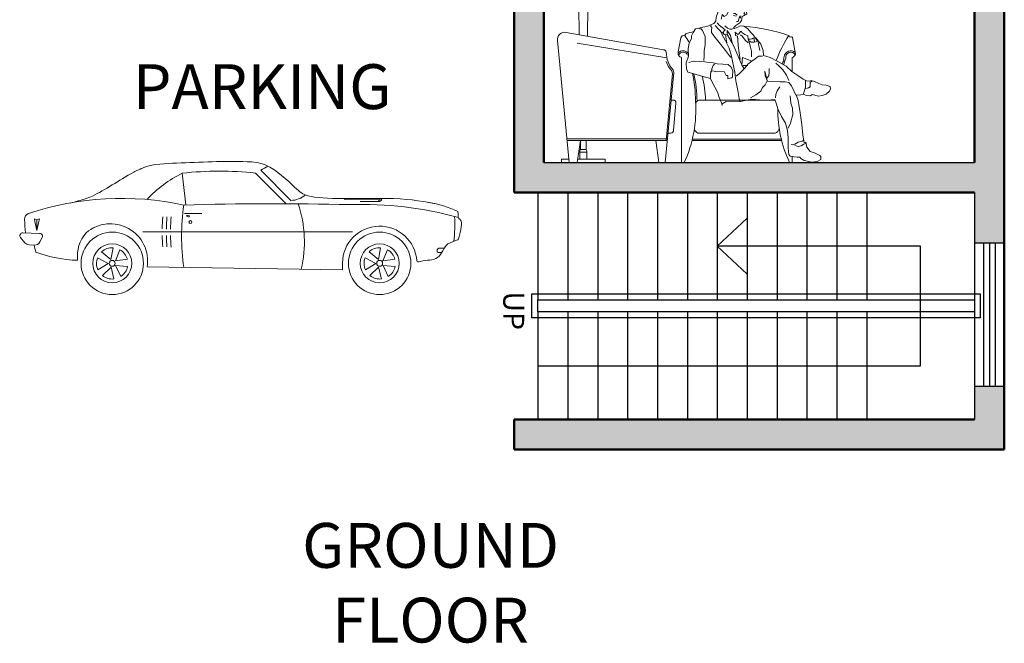
# Model space of a CAD drawing. Units: inches. Extents: x 1771 to 3025, y 319 to 889.
# Tile 1 of 35: x 1771 to 2101, y 319 to 527. Entities that reach past the tile are written whole.
import ezdxf

# ---------------------------------------------------------------- set-up
doc = ezdxf.new("R2010")
doc.units = ezdxf.units.IN
doc.header["$MEASUREMENT"] = 0
for name, color, linetype, lineweight in [('A-AREA-IDEN', 241, 'Continuous', 25), ('A-FLOR-STRS', 7, 'Continuous', 25), ('A-FURN', 8, 'Continuous', 18), ('A-GLAZ', 40, 'Continuous', 25), ('A-WALL', 7, 'Continuous', 50), ('A-WALL-PATT', 254, 'Continuous', 13), ('C-SITE-VEHC', 8, 'Continuous', 18)]:
    doc.layers.add(name, color=color, linetype=linetype, lineweight=lineweight)
doc.styles.get("Standard").update_dxf_attribs({"font": 'arial.ttf'})

# ---------------------------------------------------------------- blocks, each defined once
blk = doc.blocks.new('A$C0DCF6C46')
for p, q in [((179.4, 1650), (0, 1402.3)), ((179.4, 1650), (0, 1402.3)), ((179.4, 1650), (347.3, 1650)), ((179.4, 1650), (347.3, 1650)), ((347.3, 1650), (526.7, 1402.3)), ((347.3, 1650), (526.7, 1402.3)), ((0, 1402.3), (526.7, 1402.3)), ((0, 1402.3), (526.7, 1402.3)), ((1173.6, 1032.9), (1189.7, 1057.2)), ((1173.6, 1032.9), (1189.7, 1057.2)), ((1189.7, 1057.2), (1202.6, 1072.4)), ((1189.7, 1057.2), (1202.6, 1072.4)), ((1202.6, 1072.4), (1213.4, 1083.3)), ((1202.6, 1072.4), (1213.4, 1083.3)), ((1213.4, 1083.3), (1227.6, 1090.4)), ((1213.4, 1083.3), (1227.6, 1090.4)), ((1227.6, 1090.4), (1251, 1095.4)), ((1227.6, 1090.4), (1251, 1095.4)), ((1259.7, 1050.3), (1237.5, 1065.3)), ((1259.7, 1050.3), (1237.5, 1065.3)), ((1251, 1095.4), (1277.5, 1092)), ((1251, 1095.4), (1277.5, 1092)), ((1277.5, 1092), (1301.8, 1082.8)), ((1277.5, 1092), (1301.8, 1082.8)), ((1301.8, 1082.8), (1321.9, 1067.8)), ((1301.8, 1082.8), (1321.9, 1067.8)), ((1321.9, 1067.8), (1345.5, 1041.1)), ((1321.9, 1067.8), (1345.5, 1041.1)), ((233.4, 1042.3), (293.3, 1042.3)), ((233.4, 1042.3), (235.7, 853.7)), ((233.4, 1042.3), (293.3, 1042.3)), ((233.4, 1042.3), (235.7, 853.7)), ((244, 1051.7), (282.6, 1051.7)), ((244, 1051.7), (282.6, 1051.7)), ((293.3, 1042.3), (290.8, 843.9)), ((293.3, 1042.3), (290.8, 843.9)), ((1150.8, 970.5), (1173.6, 1032.9)), ((1150.8, 970.5), (1173.6, 1032.9)), ((1190.8, 987.7), (1188, 972.3)), ((1190.8, 987.7), (1188, 972.3)), ((1202.9, 975.4), (1190.8, 987.7)), ((1202.9, 975.4), (1190.8, 987.7)), ((1232.3, 1009.1), (1218.3, 983.7)), ((1232.3, 1009.1), (1218.3, 983.7)), ((1245.7, 1027.6), (1232.3, 1009.1)), ((1245.7, 1027.6), (1232.3, 1009.1)), ((1255.9, 1046.6), (1245.7, 1027.6)), ((1255.9, 1046.6), (1245.7, 1027.6)), ((1278.7, 1041.6), (1259.7, 1050.3)), ((1278.7, 1041.6), (1259.7, 1050.3)), ((1277.8, 994.4), (1265.6, 995)), ((1277.8, 994.4), (1265.6, 995)), ((1291.5, 983.2), (1277.8, 994.4)), ((1291.5, 983.2), (1277.8, 994.4)), ((1308.3, 1028.1), (1278.7, 1041.6)), ((1308.3, 1028.1), (1278.7, 1041.6)), ((1335.8, 1012.5), (1308.3, 1028.1)), ((1335.8, 1012.5), (1308.3, 1028.1)), ((1354.2, 991.7), (1333.4, 980.2)), ((1354.2, 991.7), (1333.4, 980.2)), ((1334, 990.3), (1338.8, 997.1)), ((1334, 990.3), (1338.8, 997.1)), ((1338.8, 997.1), (1335.8, 1012.5)), ((1338.8, 997.1), (1335.8, 1012.5)), ((1345.5, 1041.1), (1350.1, 1013.5)), ((1345.5, 1041.1), (1350.1, 1013.5)), ((1350.1, 1013.5), (1354.2, 991.7)), ((1350.1, 1013.5), (1354.2, 991.7)), ((1087.8, 908.4), (1135.7, 928.2)), ((1087.8, 908.4), (1135.7, 928.2)), ((1117, 920.9), (1113.7, 907.1)), ((1117, 920.9), (1113.7, 907.1)), ((1135.7, 928.2), (1147.4, 942.9)), ((1135.7, 928.2), (1147.4, 942.9)), ((1147.4, 942.9), (1150.8, 970.5)), ((1147.4, 942.9), (1150.8, 970.5)), ((1170.4, 917.1), (1156.8, 933.1)), ((1170.4, 917.1), (1156.8, 933.1)), ((1188, 972.3), (1182.6, 958)), ((1188, 972.3), (1182.6, 958)), ((1218.3, 983.7), (1202.9, 975.4)), ((1218.3, 983.7), (1202.9, 975.4)), ((1266, 980.7), (1284.6, 977.9)), ((1266, 980.7), (1284.6, 977.9)), ((1307.6, 932.1), (1282.5, 914.8)), ((1307.6, 932.1), (1282.5, 914.8)), ((1297.6, 940.6), (1286.8, 941.4)), ((1297.6, 940.6), (1286.8, 941.4)), ((1304.1, 966.6), (1297.6, 940.6)), ((1304.1, 966.6), (1297.6, 940.6)), ((1309.5, 977.7), (1304.1, 966.6)), ((1309.5, 977.7), (1304.1, 966.6)), ((1318.8, 948.5), (1307.6, 932.1)), ((1318.8, 948.5), (1307.6, 932.1)), ((1309.4, 969), (1312.6, 964.7)), ((1314.7, 968.9), (1309.4, 969)), ((1309.4, 969), (1312.6, 964.7)), ((1314.7, 968.9), (1309.4, 969)), ((1317.5, 977.7), (1309.5, 977.7)), ((1317.5, 977.7), (1309.5, 977.7)), ((1322.1, 963.3), (1318.8, 948.5)), ((1322.1, 963.3), (1318.8, 948.5)), ((1324.9, 973.9), (1322.1, 963.3)), ((1324.9, 973.9), (1322.1, 963.3)), ((1333.4, 980.2), (1324.9, 973.9)), ((1333.4, 980.2), (1324.9, 973.9)), ((148.7, 869.2), (799.3, 753.3)), ((148.7, 869.2), (799.3, 753.3)), ((986.5, 846.6), (995.7, 868.8)), ((986.5, 846.6), (995.7, 868.8)), ((995.7, 868.8), (1011.8, 893.6)), ((995.7, 868.8), (1011.8, 893.6)), ((1011.8, 893.6), (1033.6, 897.7)), ((1011.8, 893.6), (1033.6, 897.7)), ((1033.6, 897.7), (1060.7, 904.4)), ((1033.6, 897.7), (1060.7, 904.4)), ((1039.9, 891.8), (1050.5, 891.7)), ((1039.9, 891.8), (1050.5, 891.7)), ((1050.5, 891.7), (1058.4, 882.1)), ((1050.5, 891.7), (1058.4, 882.1)), ((1058.4, 882.1), (1076.1, 842.2)), ((1058.4, 882.1), (1076.1, 842.2)), ((1060.7, 904.4), (1087.8, 908.4)), ((1060.7, 904.4), (1087.8, 908.4)), ((1113.7, 907.1), (1121.7, 900.7)), ((1113.7, 907.1), (1121.7, 900.7)), ((1119.4, 884.3), (1119.3, 867.8)), ((1119.4, 884.3), (1119.3, 867.8)), ((1119.3, 867.8), (1135.5, 846.5)), ((1119.3, 867.8), (1135.5, 846.5)), ((1121.7, 900.7), (1119.4, 884.3)), ((1121.7, 900.7), (1119.4, 884.3)), ((1190.9, 864.1), (1144, 915.9)), ((1190.9, 864.1), (1144, 915.9)), ((1211.2, 886.7), (1170.4, 917.1)), ((1211.2, 886.7), (1170.4, 917.1)), ((1186.6, 860.4), (1212.2, 811.9)), ((1186.6, 860.4), (1212.2, 811.9)), ((1211.2, 886.7), (1190.9, 864.1)), ((1211.2, 886.7), (1190.9, 864.1)), ((1196.7, 865.6), (1204.6, 855)), ((1196.7, 865.6), (1204.6, 855)), ((1204.6, 855), (1219.4, 853.2)), ((1204.6, 855), (1219.4, 853.2)), ((1225.9, 897.6), (1208.3, 912.3)), ((1225.9, 897.6), (1208.3, 912.3)), ((1222.8, 881.9), (1223.6, 853.9)), ((1247, 848.8), (1222.8, 881.9)), ((1222.8, 881.9), (1223.6, 853.9)), ((1247, 848.8), (1222.8, 881.9)), ((1240.6, 890.8), (1225.9, 897.6)), ((1240.6, 890.8), (1225.9, 897.6)), ((1254.3, 890.2), (1240.6, 890.8)), ((1254.3, 890.2), (1240.6, 890.8)), ((1264.4, 895.9), (1254.3, 890.2)), ((1264.4, 895.9), (1254.3, 890.2)), ((1282.5, 914.8), (1267, 899.5)), ((1282.5, 914.8), (1267, 899.5)), ((1267, 899.5), (1271.7, 895.8)), ((1267, 899.5), (1271.7, 895.8)), ((1271.7, 895.8), (1295.1, 904.1)), ((1271.7, 895.8), (1295.1, 904.1)), ((1275.8, 869.8), (1284.7, 863.3)), ((1275.8, 869.8), (1284.7, 863.3)), ((1278.8, 848), (1280, 865.5)), ((1278.8, 848), (1280, 865.5)), ((1284.7, 863.3), (1296.3, 854.2)), ((1284.7, 863.3), (1296.3, 854.2)), ((1295.1, 904.1), (1310, 911.9)), ((1295.1, 904.1), (1310, 911.9)), ((1296.3, 854.2), (1303.8, 861.6)), ((1296.3, 854.2), (1303.8, 861.6)), ((1303.8, 861.6), (1313.5, 875.8)), ((1303.8, 861.6), (1313.5, 875.8)), ((1310, 911.9), (1334.4, 909.6)), ((1310, 911.9), (1334.4, 909.6)), ((1313.5, 875.8), (1318.8, 876.9)), ((1313.5, 875.8), (1318.8, 876.9)), ((1318.8, 876.9), (1321.4, 867.3)), ((1318.8, 876.9), (1321.4, 867.3)), ((1321.4, 867.3), (1342.5, 854.4)), ((1321.4, 867.3), (1342.5, 854.4)), ((1334.4, 909.6), (1359.2, 894.6)), ((1334.4, 909.6), (1359.2, 894.6)), ((1359.2, 894.6), (1384, 866.8)), ((1359.2, 894.6), (1384, 866.8)), ((1384, 866.8), (1396.6, 853.4)), ((1384, 866.8), (1396.6, 853.4)), ((167.7, 0), (90.2, 815.3)), ((167.7, 0), (90.2, 815.3)), ((821.8, 697.8), (222.3, 796.3)), ((821.8, 697.8), (222.3, 796.3)), ((915.2, 833), (897.4, 738.2)), ((915.2, 833), (897.4, 738.2)), ((966.3, 773.5), (970.2, 796.3)), ((966.3, 773.5), (970.2, 796.3)), ((970.2, 796.3), (984.8, 829.6)), ((970.2, 796.3), (984.8, 829.6)), ((984.8, 829.6), (986.5, 846.6)), ((984.8, 829.6), (986.5, 846.6)), ((1076.1, 842.2), (1077.8, 785.9)), ((1076.1, 842.2), (1077.8, 785.9)), ((1135.5, 846.5), (1162.3, 812.3)), ((1135.5, 846.5), (1162.3, 812.3)), ((1162.3, 812.3), (1187.5, 779.8)), ((1162.3, 812.3), (1187.5, 779.8)), ((1212.2, 811.9), (1236.7, 763.5)), ((1212.2, 811.9), (1236.7, 763.5)), ((1213.6, 851.7), (1221.1, 799.1)), ((1213.6, 851.7), (1221.1, 799.1)), ((1223.6, 853.9), (1255.4, 801.3)), ((1223.6, 853.9), (1255.4, 801.3)), ((1257.2, 799.9), (1247, 848.8)), ((1257.2, 799.9), (1247, 848.8)), ((1275.4, 760.5), (1257.2, 799.9)), ((1275.4, 760.5), (1257.2, 799.9)), ((1293.6, 844.7), (1278.8, 848)), ((1293.6, 844.7), (1278.8, 848)), ((1293.9, 818.2), (1293.6, 844.7)), ((1293.9, 818.2), (1293.6, 844.7)), ((1296.3, 781), (1293.9, 818.2)), ((1296.3, 781), (1293.9, 818.2)), ((1325.9, 840.7), (1312.2, 852)), ((1325.9, 840.7), (1312.2, 852)), ((1343.2, 816.2), (1325.9, 840.7)), ((1343.2, 816.2), (1325.9, 840.7)), ((1342.5, 854.4), (1362, 845.8)), ((1342.5, 854.4), (1362, 845.8)), ((1364.9, 799.6), (1343.2, 816.2)), ((1364.9, 799.6), (1343.2, 816.2)), ((1362, 845.8), (1365, 822.9)), ((1362, 845.8), (1365, 822.9)), ((1376.2, 822.8), (1365, 822.9)), ((1365, 822.9), (1371.3, 804.3)), ((1376.2, 822.8), (1365, 822.9)), ((1365, 822.9), (1371.3, 804.3)), ((1371.3, 804.3), (1380.5, 770.8)), ((1371.3, 804.3), (1380.5, 770.8)), ((1384, 803.7), (1372.4, 811.7)), ((1384, 803.7), (1372.4, 811.7)), ((1390.5, 825.9), (1376.2, 822.8)), ((1390.5, 825.9), (1376.2, 822.8)), ((1403.6, 803.5), (1384, 803.7)), ((1403.6, 803.5), (1384, 803.7)), ((1401.2, 832.2), (1390.5, 825.9)), ((1401.2, 832.2), (1390.5, 825.9)), ((1396.6, 853.4), (1411.8, 831)), ((1396.6, 853.4), (1411.8, 831)), ((1405.2, 808.3), (1401.2, 832.2)), ((1405.2, 808.3), (1401.2, 832.2)), ((1423.8, 807.1), (1403.6, 803.5)), ((1423.8, 807.1), (1403.6, 803.5)), ((1411.8, 831), (1422.3, 818.2)), ((1411.8, 831), (1422.3, 818.2)), ((1414.4, 832.1), (1447.5, 790.5)), ((1414.4, 832.1), (1447.5, 790.5)), ((1422.3, 818.2), (1423.8, 807.1)), ((1422.3, 818.2), (1423.8, 807.1)), ((1431.7, 801.7), (1440.8, 748.6)), ((1431.7, 801.7), (1440.8, 748.6)), ((1447.5, 790.5), (1463.6, 748.4)), ((1447.5, 790.5), (1463.6, 748.4)), ((1637.6, 846.8), (1643.1, 837.5)), ((1637.6, 846.8), (1643.1, 837.5)), ((1680.1, 723.7), (1660.3, 834.6)), ((1680.1, 723.7), (1660.3, 834.6)), ((816.5, 736.2), (823.2, 687.2)), ((816.5, 736.2), (823.2, 687.2)), ((963, 758.2), (966.3, 773.5)), ((963, 758.2), (966.3, 773.5)), ((965.8, 711), (963, 758.2)), ((965.8, 711), (963, 758.2)), ((1071.1, 747.3), (1070.3, 709.1)), ((1071.1, 747.3), (1070.3, 709.1)), ((1077.8, 785.9), (1071.1, 747.3)), ((1077.8, 785.9), (1071.1, 747.3)), ((1187.5, 779.8), (1212.2, 747.2)), ((1187.5, 779.8), (1212.2, 747.2)), ((1212.2, 747.2), (1239, 712)), ((1212.2, 747.2), (1239, 712)), ((1236.7, 763.5), (1253.3, 709.8)), ((1236.7, 763.5), (1253.3, 709.8)), ((1294.7, 714.7), (1275.4, 760.5)), ((1294.7, 714.7), (1275.4, 760.5)), ((1304.4, 731.6), (1296.3, 781)), ((1304.4, 731.6), (1296.3, 781)), ((1310.9, 687.6), (1304.4, 731.6)), ((1310.9, 687.6), (1304.4, 731.6)), ((1380.5, 770.8), (1387.2, 743.7)), ((1380.5, 770.8), (1387.2, 743.7)), ((1387.2, 743.7), (1387.1, 723)), ((1387.2, 743.7), (1387.1, 723)), ((1463.6, 748.4), (1467.1, 713.4)), ((1463.6, 748.4), (1467.1, 713.4)), ((816.1, 675.1), (831.6, 638.4)), ((816.1, 675.1), (831.6, 638.4)), ((823.2, 687.2), (840.7, 645.7)), ((823.2, 687.2), (840.7, 645.7)), ((919.8, 701.9), (919.8, 0)), ((919.8, 701.9), (919.8, 0)), ((949, 665.5), (965.8, 711)), ((949, 665.5), (965.8, 711)), ((952.4, 624.6), (949, 665.5)), ((952.4, 624.6), (949, 665.5)), ((968.1, 667.4), (995.8, 675.7)), ((968.1, 667.4), (995.8, 675.7)), ((995.8, 675.7), (1036.1, 673.3)), ((995.8, 675.7), (1036.1, 673.3)), ((1036.1, 673.3), (1074.2, 672.4)), ((1036.1, 673.3), (1074.2, 672.4)), ((1070.3, 709.1), (1067.4, 681)), ((1070.3, 709.1), (1067.4, 681)), ((1074.2, 672.4), (1099.7, 668.5)), ((1074.2, 672.4), (1099.7, 668.5)), ((1099.7, 668.5), (1130.9, 665.6)), ((1099.7, 668.5), (1130.9, 665.6)), ((1130.9, 665.6), (1156.4, 659.6)), ((1130.9, 665.6), (1156.4, 659.6)), ((1156.4, 659.6), (1194, 656.7)), ((1156.4, 659.6), (1194, 656.7)), ((1239, 712), (1250, 700.8)), ((1239, 712), (1250, 700.8)), ((1253.3, 709.8), (1262, 665.7)), ((1253.3, 709.8), (1262, 665.7)), ((1262, 665.7), (1274.2, 603)), ((1262, 665.7), (1274.2, 603)), ((1319.7, 657.3), (1294.7, 714.7)), ((1319.7, 657.3), (1294.7, 714.7)), ((1325.9, 701.8), (1321.2, 649.3)), ((1325.9, 701.8), (1321.2, 649.3)), ((1387.8, 675.8), (1325.9, 701.8)), ((1387.8, 675.8), (1325.9, 701.8)), ((1342.9, 632.7), (1362.7, 657.4)), ((1342.9, 632.7), (1362.7, 657.4)), ((1362.7, 657.4), (1387.8, 675.8)), ((1362.7, 657.4), (1387.8, 675.8)), ((1387.1, 723), (1385.3, 706.1)), ((1387.1, 723), (1385.3, 706.1)), ((1387.8, 675.8), (1410.2, 693.1)), ((1387.8, 675.8), (1410.2, 693.1)), ((1410.2, 693.1), (1433.6, 709.9)), ((1410.2, 693.1), (1433.6, 709.9)), ((1433.6, 709.9), (1459.6, 709.7)), ((1433.6, 709.9), (1459.6, 709.7)), ((1467.1, 713.4), (1510.5, 701.4)), ((1467.1, 713.4), (1510.5, 701.4)), ((1510.5, 701.4), (1562.3, 673.9)), ((1510.5, 701.4), (1562.3, 673.9)), ((1569.5, 644.7), (1548.9, 662.4)), ((1569.5, 644.7), (1548.9, 662.4)), ((1562.3, 673.9), (1616.6, 642.7)), ((1562.3, 673.9), (1616.6, 642.7)), ((1656.8, 701.9), (1656.8, 607.1)), ((1656.8, 701.9), (1656.8, 607.1)), ((867.8, 600.3), (810.7, 0)), ((867.8, 600.3), (810.7, 0)), ((858.7, 592.9), (816.6, 146.6)), ((858.7, 592.9), (816.6, 146.6)), ((831.6, 638.4), (853.4, 612.1)), ((831.6, 638.4), (853.4, 612.1)), ((840.7, 645.7), (862.6, 619.4)), ((840.7, 645.7), (862.6, 619.4)), ((853.4, 612.1), (858.7, 592.9)), ((853.4, 612.1), (858.7, 592.9)), ((862.6, 619.4), (867.8, 600.3)), ((862.6, 619.4), (867.8, 600.3)), ((961.2, 603.3), (952.4, 624.6)), ((961.2, 603.3), (952.4, 624.6)), ((994.1, 595.1), (961.2, 603.3)), ((994.1, 595.1), (961.2, 603.3)), ((1053.9, 576.6), (994.1, 595.1)), ((1053.9, 576.6), (994.1, 595.1)), ((1111.3, 595.2), (1113.2, 565.5)), ((1111.3, 595.2), (1113.2, 565.5)), ((1115.1, 607.9), (1115, 596.8)), ((1115.1, 607.9), (1115, 596.8)), ((1128.9, 611.5), (1115.1, 607.9)), ((1128.9, 611.5), (1115.1, 607.9)), ((1115.6, 599.4), (1119.9, 607.9)), ((1115.6, 599.4), (1119.9, 607.9)), ((1119.9, 607.9), (1120.6, 625.4)), ((1119.9, 607.9), (1120.6, 625.4)), ((1120.6, 625.4), (1130.3, 647.1)), ((1120.6, 625.4), (1130.3, 647.1)), ((1154.9, 605), (1128.9, 611.5)), ((1154.9, 605), (1128.9, 611.5)), ((1130.3, 647.1), (1138.8, 656.6)), ((1130.3, 647.1), (1138.8, 656.6)), ((1202.6, 606.7), (1154.9, 605)), ((1202.6, 606.7), (1154.9, 605)), ((1194, 656.7), (1230, 653.7)), ((1194, 656.7), (1230, 653.7)), ((1217.8, 581.7), (1202.6, 606.7)), ((1217.8, 581.7), (1202.6, 606.7)), ((1230, 653.7), (1248, 637.7)), ((1230, 653.7), (1248, 637.7)), ((1248, 637.7), (1261.6, 613.2)), ((1248, 637.7), (1261.6, 613.2)), ((1261.6, 613.2), (1259.1, 569.7)), ((1261.6, 613.2), (1259.1, 569.7)), ((1274.2, 603), (1280.6, 545.6)), ((1274.2, 603), (1280.6, 545.6)), ((1284.6, 575.8), (1304.9, 592.7)), ((1284.6, 575.8), (1304.9, 592.7)), ((1304.9, 592.7), (1325.7, 613.7)), ((1304.9, 592.7), (1325.7, 613.7)), ((1321.2, 649.3), (1340.1, 623.1)), ((1321.2, 649.3), (1340.1, 623.1)), ((1325.7, 613.7), (1342.9, 632.7)), ((1325.7, 613.7), (1342.9, 632.7)), ((1361.5, 647.4), (1329.7, 647.6)), ((1361.5, 647.4), (1329.7, 647.6)), ((1475.8, 608.8), (1478.2, 578)), ((1491.8, 546.1), (1475.8, 608.8)), ((1475.8, 608.8), (1478.2, 578)), ((1491.8, 546.1), (1475.8, 608.8)), ((1501, 578.9), (1503.4, 603.8)), ((1501, 578.9), (1503.4, 603.8)), ((1503.4, 603.8), (1505.1, 628.7)), ((1503.4, 603.8), (1505.1, 628.7)), ((1595.2, 618), (1569.5, 644.7)), ((1595.2, 618), (1569.5, 644.7)), ((1618.8, 582.8), (1595.2, 618)), ((1618.8, 582.8), (1595.2, 618)), ((1616.6, 642.7), (1655.6, 607.9)), ((1616.6, 642.7), (1655.6, 607.9)), ((1655.6, 607.9), (1695.2, 580.6)), ((1655.6, 607.9), (1695.2, 580.6)), ((1112.1, 561.3), (1053.9, 576.6)), ((1112.1, 561.3), (1053.9, 576.6)), ((1128.3, 528.3), (1112.1, 561.3)), ((1128.3, 528.3), (1112.1, 561.3)), ((1142.4, 502.7), (1128.3, 528.3)), ((1142.4, 502.7), (1128.3, 528.3)), ((1228.9, 581.6), (1217.8, 581.7)), ((1228.9, 581.6), (1217.8, 581.7)), ((1228.2, 558.8), (1228.9, 581.6)), ((1228.2, 558.8), (1228.9, 581.6)), ((1252.7, 566), (1228.2, 558.8)), ((1252.7, 566), (1228.2, 558.8)), ((1259.1, 569.7), (1252.7, 566)), ((1259.1, 569.7), (1252.7, 566)), ((1280.6, 545.6), (1294.5, 479.8)), ((1280.6, 545.6), (1294.5, 479.8)), ((1478.2, 578), (1493.9, 543.4)), ((1478.2, 578), (1493.9, 543.4)), ((1478.3, 517.6), (1491.8, 546.1)), ((1478.3, 517.6), (1491.8, 546.1)), ((1489.2, 562.6), (1501, 578.9)), ((1489.2, 562.6), (1501, 578.9)), ((1493.9, 543.4), (1527.3, 540.5)), ((1493.9, 543.4), (1527.3, 540.5)), ((1527.3, 540.5), (1578.2, 538)), ((1527.3, 540.5), (1578.2, 538)), ((1578.2, 538), (1610.5, 537.7)), ((1578.2, 538), (1610.5, 537.7)), ((1610.5, 537.7), (1634.4, 534.9)), ((1610.5, 537.7), (1634.4, 534.9)), ((1635.5, 547.1), (1618.8, 582.8)), ((1635.5, 547.1), (1618.8, 582.8)), ((1634.4, 534.9), (1652.2, 511.4)), ((1634.4, 534.9), (1652.2, 511.4)), ((1695.2, 580.6), (1732.1, 555.4)), ((1695.2, 580.6), (1732.1, 555.4)), ((1732.1, 555.4), (1753.8, 546.2)), ((1732.1, 555.4), (1753.8, 546.2)), ((1747.8, 525.5), (1746.4, 548.4)), ((1747.8, 525.5), (1746.4, 548.4)), ((1753.8, 546.2), (1776.6, 543.9)), ((1753.8, 546.2), (1776.6, 543.9)), ((1776.6, 543.9), (1784.6, 547)), ((1776.6, 543.9), (1784.6, 547)), ((1788.3, 543.8), (1777, 533.3)), ((1788.3, 543.8), (1777, 533.3)), ((1777, 533.3), (1777, 522.1)), ((1777, 533.3), (1777, 522.1)), ((1784.6, 547), (1807.3, 541.5)), ((1784.6, 547), (1807.3, 541.5)), ((1807.3, 541.5), (1836.4, 528.5)), ((1807.3, 541.5), (1836.4, 528.5)), ((1836.4, 528.5), (1857.6, 518.8)), ((1836.4, 528.5), (1857.6, 518.8)), ((1162.3, 464.9), (1142.4, 502.7)), ((1162.3, 464.9), (1142.4, 502.7)), ((1170.5, 433.5), (1162.3, 464.9)), ((1170.5, 433.5), (1162.3, 464.9)), ((1294.5, 479.8), (1303.6, 427.7)), ((1294.5, 479.8), (1303.6, 427.7)), ((1415.7, 451.8), (1447.7, 477)), ((1415.7, 451.8), (1447.7, 477)), ((1447.7, 477), (1460.7, 501.8)), ((1447.7, 477), (1460.7, 501.8)), ((1460.7, 501.8), (1478.3, 517.6)), ((1460.7, 501.8), (1478.3, 517.6)), ((1547.8, 455), (1556.5, 478.8)), ((1547.8, 455), (1556.5, 478.8)), ((1556.5, 478.8), (1575.3, 505.7)), ((1556.5, 478.8), (1575.3, 505.7)), ((1652.2, 511.4), (1671, 474.2)), ((1652.2, 511.4), (1671, 474.2)), ((1671, 474.2), (1681.4, 448.6)), ((1671, 474.2), (1681.4, 448.6)), ((1732.4, 458.3), (1740, 481)), ((1732.4, 458.3), (1740, 481)), ((1740, 481), (1747.1, 502.7)), ((1740, 481), (1747.1, 502.7)), ((1747.1, 502.7), (1747.8, 525.5)), ((1747.1, 502.7), (1747.8, 525.5)), ((1766.2, 498.3), (1749.2, 494.8)), ((1766.2, 498.3), (1749.2, 494.8)), ((1776.8, 504.6), (1766.2, 498.3)), ((1776.8, 504.6), (1766.2, 498.3)), ((1777, 522.1), (1776.8, 504.6)), ((1777, 522.1), (1776.8, 504.6)), ((1857.6, 518.8), (1884.1, 516)), ((1857.6, 518.8), (1884.1, 516)), ((1884.1, 516), (1912.1, 507.8)), ((1884.1, 516), (1912.1, 507.8)), ((1906, 476.6), (1884.1, 456)), ((1906, 476.6), (1884.1, 456)), ((1913, 492.4), (1906, 476.6)), ((1913, 492.4), (1906, 476.6)), ((1912.1, 507.8), (1913, 492.4)), ((1912.1, 507.8), (1913, 492.4)), ((862, 416.6), (851.4, 416.6)), ((862, 416.6), (851.4, 416.6)), ((882, 396.6), (866.1, 216.6)), ((882, 396.6), (866.1, 216.6)), ((1033.5, 416.6), (1544.9, 416.6)), ((1033.5, 416.6), (1544.9, 416.6)), ((1186.7, 397.9), (1170.5, 433.5)), ((1186.7, 397.9), (1170.5, 433.5)), ((1189.7, 380.9), (1186.7, 397.9)), ((1189.7, 380.9), (1186.7, 397.9)), ((1217.5, 406.6), (1189.8, 391.5)), ((1217.5, 406.6), (1189.8, 391.5)), ((1262, 404.2), (1217.5, 406.6)), ((1262, 404.2), (1217.5, 406.6)), ((1315.1, 406.4), (1262, 404.2)), ((1315.1, 406.4), (1262, 404.2)), ((1303.6, 427.7), (1308.2, 407)), ((1303.6, 427.7), (1308.2, 407)), ((1351.8, 416.7), (1315.1, 406.4)), ((1351.8, 416.7), (1315.1, 406.4)), ((1388.4, 423.3), (1351.8, 416.7)), ((1388.4, 423.3), (1351.8, 416.7)), ((1379, 432.4), (1415.7, 451.8)), ((1379, 432.4), (1415.7, 451.8)), ((1440.4, 418.1), (1388.4, 423.3)), ((1440.4, 418.1), (1388.4, 423.3)), ((1490.2, 415.6), (1440.4, 418.1)), ((1490.2, 415.6), (1440.4, 418.1)), ((1542.2, 420.5), (1490.2, 415.6)), ((1542.2, 420.5), (1490.2, 415.6)), ((1552.6, 389.1), (1542.2, 420.5)), ((1552.6, 389.1), (1542.2, 420.5)), ((1546.6, 431.1), (1547.8, 455)), ((1546.6, 431.1), (1547.8, 455)), ((1645.3, 444.1), (1649.7, 395.3)), ((1645.3, 444.1), (1649.7, 395.3)), ((1649.7, 395.3), (1660.1, 361.8)), ((1649.7, 395.3), (1660.1, 361.8)), ((1683.6, 450.7), (1697.6, 414)), ((1699.5, 448.5), (1683.6, 450.7)), ((1683.6, 450.7), (1697.6, 414)), ((1699.5, 448.5), (1683.6, 450.7)), ((1697.6, 414), (1703.2, 388)), ((1697.6, 414), (1703.2, 388)), ((1715.9, 452.6), (1699.5, 448.5)), ((1715.9, 452.6), (1699.5, 448.5)), ((1736.6, 455.1), (1715.9, 452.6)), ((1736.6, 455.1), (1715.9, 452.6)), ((1750.9, 447.5), (1736.6, 455.1)), ((1750.9, 447.5), (1736.6, 455.1)), ((1780.1, 445.7), (1750.9, 447.5)), ((1780.1, 445.7), (1750.9, 447.5)), ((1792.3, 453.6), (1780.1, 445.7)), ((1792.3, 453.6), (1780.1, 445.7)), ((1833.1, 442.1), (1792.3, 453.6)), ((1833.1, 442.1), (1792.3, 453.6)), ((1859.1, 446.7), (1833.1, 442.1)), ((1859.1, 446.7), (1833.1, 442.1)), ((1884.1, 456), (1859.1, 446.7)), ((1884.1, 456), (1859.1, 446.7)), ((1189.8, 391.5), (1189.7, 380.9)), ((1189.8, 391.5), (1189.7, 380.9)), ((1563, 357.2), (1552.6, 389.1)), ((1563, 357.2), (1552.6, 389.1)), ((1585.9, 307.2), (1563, 357.2)), ((1585.9, 307.2), (1563, 357.2)), ((1660.1, 361.8), (1662.9, 319.9)), ((1660.1, 361.8), (1662.9, 319.9)), ((1703.2, 388), (1711.8, 331.7)), ((1703.2, 388), (1711.8, 331.7)), ((1711.8, 331.7), (1721.8, 252.6)), ((1711.8, 331.7), (1721.8, 252.6)), ((1612.6, 261.4), (1585.9, 307.2)), ((1612.6, 261.4), (1585.9, 307.2)), ((1645.5, 263.2), (1632, 228.9)), ((1645.5, 263.2), (1632, 228.9)), ((1662.9, 319.9), (1645.5, 263.2)), ((1662.9, 319.9), (1645.5, 263.2)), ((1625.5, 214.1), (1612.6, 261.4)), ((1625.5, 214.1), (1612.6, 261.4)), ((1629.9, 164.2), (1625.5, 214.1)), ((1629.9, 164.2), (1625.5, 214.1)), ((1721.8, 252.6), (1729.7, 181.9)), ((1721.8, 252.6), (1729.7, 181.9)), ((825, 157.1), (152.8, 157.1)), ((825, 157.1), (152.8, 157.1)), ((825, 146.6), (153.8, 146.6)), ((825, 146.6), (153.8, 146.6)), ((243.8, 146.6), (221.9, 0)), ((243.8, 146.6), (221.9, 0)), ((244.6, 146.6), (245.3, 86.3)), ((244.6, 146.6), (245.3, 86.3)), ((282.1, 146.6), (281.3, 86.3)), ((282.1, 146.6), (281.3, 86.3)), ((746.4, 146.6), (768.4, 0)), ((746.4, 146.6), (768.4, 0)), ((846.1, 196.6), (829.9, 196.6)), ((846.1, 196.6), (829.9, 196.6)), ((989.7, 156.6), (1587.6, 156.6)), ((989.7, 156.6), (1587.6, 156.6)), ((989.7, 146.6), (1587.6, 146.6)), ((989.7, 146.6), (1587.6, 146.6)), ((1028.1, 196.6), (1544.2, 196.6)), ((1028.1, 196.6), (1544.2, 196.6)), ((1630.1, 127.6), (1629.9, 164.2)), ((1630.1, 127.6), (1629.9, 164.2)), ((1698.1, 135), (1675.7, 123)), ((1698.1, 135), (1675.7, 123)), ((1724.1, 142.7), (1698.1, 135)), ((1724.1, 142.7), (1698.1, 135)), ((1737.4, 151.1), (1724.1, 142.7)), ((1737.4, 151.1), (1724.1, 142.7)), ((1729.7, 181.9), (1734.7, 143.7)), ((1729.7, 181.9), (1734.7, 143.7)), ((1734.7, 143.7), (1737.8, 131)), ((1734.7, 143.7), (1737.8, 131)), ((1737.8, 131), (1747.9, 135.7)), ((1737.8, 131), (1747.9, 135.7)), ((1747.9, 135.7), (1755.6, 101.1)), ((1747.9, 135.7), (1755.6, 101.1)), ((234.6, 85), (244.2, 85)), ((234.6, 85), (244.2, 85)), ((236.8, 100), (245.2, 100)), ((236.8, 100), (245.2, 100)), ((239.8, 68.3), (239.8, 22.5)), ((239.8, 68.3), (286.9, 68.3)), ((239.8, 68.3), (239.8, 22.5)), ((239.8, 68.3), (286.9, 68.3)), ((245.3, 86.3), (281.3, 86.3)), ((245.3, 86.3), (281.3, 86.3)), ((286.9, 68.3), (286.9, 22.5)), ((286.9, 68.3), (286.9, 22.5)), ((1631, 102.1), (1630.1, 127.6)), ((1631, 102.1), (1630.1, 127.6)), ((1632.3, 70.8), (1631, 102.1)), ((1632.3, 70.8), (1631, 102.1)), ((1635.9, 52.2), (1632.3, 70.8)), ((1635.9, 52.2), (1632.3, 70.8)), ((1661.3, 116.7), (1650.2, 119.5)), ((1661.3, 116.7), (1650.2, 119.5)), ((1675.7, 123), (1661.3, 116.7)), ((1675.7, 123), (1661.3, 116.7)), ((1701, 106.3), (1675.6, 113.9)), ((1701, 106.3), (1675.6, 113.9)), ((1717, 111.5), (1701, 106.3)), ((1717, 111.5), (1701, 106.3)), ((1735.1, 122.5), (1717, 111.5)), ((1735.1, 122.5), (1717, 111.5)), ((1747.3, 126.1), (1735.1, 122.5)), ((1747.3, 126.1), (1735.1, 122.5)), ((1755.6, 101.1), (1777.7, 72.3)), ((1755.6, 101.1), (1777.7, 72.3)), ((1777.7, 72.3), (1806.8, 63.6)), ((1777.7, 72.3), (1806.8, 63.6)), ((116.8, 22.5), (116.8, 0)), ((116.8, 22.5), (165.6, 22.5)), ((116.8, 22.5), (116.8, 0)), ((116.8, 22.5), (165.6, 22.5)), ((225.2, 22.5), (409.9, 22.5)), ((225.2, 22.5), (409.9, 22.5)), ((409.9, 22.5), (409.9, 0)), ((409.9, 22.5), (409.9, 0)), ((1645.4, 43.1), (1635.9, 52.2)), ((1645.4, 43.1), (1635.9, 52.2)), ((1669.2, 38.7), (1645.4, 43.1)), ((1669.2, 38.7), (1645.4, 43.1)), ((1656.8, 41), (1656.8, 0)), ((1656.8, 41), (1656.8, 0)), ((1691.4, 35.3), (1669.2, 38.7)), ((1691.4, 35.3), (1669.2, 38.7)), ((1709, 35.2), (1691.4, 35.3)), ((1709, 35.2), (1691.4, 35.3)), ((1715.3, 26.6), (1709, 35.2)), ((1715.3, 26.6), (1709, 35.2)), ((1738, 13.7), (1715.3, 26.6)), ((1738, 13.7), (1715.3, 26.6)), ((1789.3, 2.7), (1738, 13.7)), ((1789.3, 2.7), (1738, 13.7)), ((1824.4, 6.7), (1789.3, 2.7)), ((1824.4, 6.7), (1789.3, 2.7)), ((1806.8, 63.6), (1841.7, 47.4)), ((1806.8, 63.6), (1841.7, 47.4)), ((1849.4, 20.8), (1824.4, 6.7)), ((1849.4, 20.8), (1824.4, 6.7)), ((1841.7, 47.4), (1849.6, 39.4)), ((1841.7, 47.4), (1849.6, 39.4)), ((1849.6, 39.4), (1849.4, 20.8)), ((1849.6, 39.4), (1849.4, 20.8)), ((116.8, 0), (409.9, 0)), ((116.8, 0), (409.9, 0)), ((919.8, 0), (937.1, 0)), ((919.8, 0), (937.1, 0)), ((1639.4, 0), (1656.8, 0)), ((1639.4, 0), (1656.8, 0))]:
    blk.add_line(p, q)
for centre, radius, start, end in [((232.2, 1398.2), 40.9, 298.59102, 4.78014), ((232.2, 1398.2), 40.9, 298.59102, 4.78014), ((232.2, 1398.2), 48.9, 302.77937, 4.78014), ((232.2, 1398.2), 48.9, 302.77937, 4.78014), ((374.6, 1328.2), 127.4, 164.50889, 205.7991), ((374.6, 1328.2), 127.4, 164.50889, 205.7991), ((374.6, 1328.2), 119.4, 166.02791, 204.23404), ((374.6, 1328.2), 119.4, 166.02791, 204.23404), ((251.6, 1244.5), 29.4, 308.7103, 73.80332), ((251.6, 1244.5), 29.4, 308.7103, 73.80332), ((251.6, 1244.5), 37.4, 311.19288, 67.98216), ((251.6, 1244.5), 37.4, 311.19288, 67.98216), ((395.6, 1149.4), 144.8, 150.11503, 204.77508), ((395.6, 1149.4), 144.8, 150.11503, 204.77508), ((395.6, 1149.4), 136.8, 150.70049, 204.76275), ((395.6, 1149.4), 136.8, 150.70049, 204.76275), ((231.9, 1073.6), 35.6, 321.99565, 25.2261), ((231.9, 1073.6), 35.6, 321.99565, 25.2261), ((231.9, 1073.6), 43.6, 329.69607, 25.18201), ((231.9, 1073.6), 43.6, 329.69607, 25.18201), ((246.1, 1038.6), 13.2, 98.80515, 163.92366), ((246.1, 1038.6), 13.2, 98.80515, 163.92366), ((280.6, 1038.6), 13.2, 16.07634, 81.19485), ((280.6, 1038.6), 13.2, 16.07634, 81.19485), ((139.9, 820), 50, 79.89119, 185.43368), ((139.9, 820), 50, 79.89119, 185.43368), ((1047.8, 778.9), 128.2, 140.79379, 148.04958), ((1047.8, 778.9), 128.2, 140.79379, 148.04958), ((1273.4, -169.1), 1079.2, 104.70187, 107.52711), ((1273.4, -169.1), 1079.2, 104.70187, 107.52711), ((1273.4, -169.1), 1079.2, 70.27897, 86.636), ((1273.4, -169.1), 1079.2, 70.27897, 86.636), ((933.1, 829.6), 18.2, 70.94115, 169.10122), ((933.1, 829.6), 18.2, 70.94115, 169.10122), ((241, 385.5), 838.8, 30.00421, 33.52274), ((241, 385.5), 838.8, 30.00421, 33.52274), ((2335, 385.5), 838.2, 146.55548, 159.4144), ((2335, 385.5), 838.2, 146.55548, 159.4144), ((1650.3, 825), 14.4, 42.1894, 120.22739), ((1650.3, 825), 14.4, 42.1894, 120.22739), ((796.6, 733.4), 20, 7.85836, 82.48429), ((796.6, 733.4), 20, 7.85836, 82.48429), ((923.6, 729.2), 27.6, 161.10495, 262.17796), ((923.6, 729.2), 27.6, 161.10495, 262.17796), ((929, 702.9), 43.5, 37.81347, 139.32094), ((929, 702.9), 43.5, 37.81347, 139.32094), ((929, 702.9), 33.5, 26.38545, 153.12764), ((929, 702.9), 33.5, 26.38545, 153.12764), ((1647.6, 702.9), 43.5, 45.07885, 176.31976), ((1647.6, 702.9), 43.5, 45.07885, 176.31976), ((1647.6, 702.9), 33.5, 26.87236, 191.36885), ((1647.6, 702.9), 33.5, 26.87236, 191.36885), ((1653, 729.2), 27.6, 277.82204, 348.41793), ((1653, 729.2), 27.6, 277.82204, 348.41793), ((2392.2, 407.9), 838, 160.74027, 162.71962), ((2392.2, 407.9), 838, 160.74027, 162.71962), ((2420.3, 406.7), 856.1, 160.22448, 163.33322), ((2420.3, 406.7), 856.1, 160.22448, 163.33322), ((1639.4, 689.8), 38.7, 155.75278, 188.14412), ((1639.4, 689.8), 38.7, 155.75278, 188.14412), ((156.3, 406.7), 856.1, 0.18203, 12.76605), ((156.3, 406.7), 856.1, 0.18203, 12.76605), ((176.7, 406.6), 845.7, 0.16174, 12.7147), ((176.7, 406.6), 845.7, 0.16174, 12.7147), ((241, 385.5), 838.8, 2.12384, 13.09126), ((241, 385.5), 838.8, 2.12384, 13.09126), ((862, 396.6), 20, 0, 90), ((862, 396.6), 20, 0, 90), ((178.3, 351), 836.1, 335.17556, 4.00033), ((178.3, 351), 836.1, 335.17556, 4.00033), ((1052.6, 376.5), 44.4, 115.39182, 154.20701), ((1052.6, 376.5), 44.4, 115.39182, 154.20701), ((2398.3, 351), 836.1, 179.42086, 204.82444), ((2398.3, 351), 836.1, 179.42086, 204.82444), ((846.1, 216.6), 20, 270, 0), ((846.1, 216.6), 20, 270, 0), ((1045.3, 237.5), 44.4, 202.02539, 247.09465), ((1045.3, 237.5), 44.4, 202.02539, 247.09465), ((1529.6, 238.5), 44.4, 289.11707, 341.80542), ((1529.6, 238.5), 44.4, 289.11707, 341.80542), ((262.7, 71.1), 23.1, 138.77414, 186.87979), ((262.7, 71.1), 23.1, 138.77414, 186.87979), ((263.9, 71.1), 23.1, 353.12021, 41.22586), ((263.9, 71.1), 23.1, 353.12021, 41.22586)]:
    blk.add_arc(centre, radius, start, end)
blk = doc.blocks.new('A$C4223307F')
blk.add_line((768.4, 0), (810.7, 0))
blk.add_blockref('A$C0DCF6C46', (0, 0))
blk = doc.blocks.new('A$C061F63B6')
blk.add_blockref('A$C4223307F', (0, 0))
blk = doc.blocks.new('*U17')
for p, q in [((72.93, 40.23), (85.8, 53.18)), ((75, 38.82), (88.08, 51.97)), ((119.39, 51.91), (117.92, 38.32)), ((50.13, 41.06), (34.31, 40.98)), ((43.26, 39.85), (35.15, 39.78)), ((35.3, 40.46), (50.13, 40.62)), ((111.09, 34.73), (118.48, 34.64)), ((46.65, 26.83), (136.29, 26.77)), ((180.37, 26.17), (187.51, 26.41)), ((179.3, 24.35), (180.25, 22.49)), ((182.62, 21.14), (184.91, 21.28)), ((186.68, 22.17), (188.51, 24.37)), ((7.45, 19.78), (9.74, 19.8)), ((9.76, 17.93), (8.53, 17.92)), ((10.37, 19.19), (10.38, 18.56)), ((50.87, 13.52), (50.91, 10.52))]:
    blk.add_line(p, q)
for points in [[(35.31, 39.93), (35.3, 40.27, 0.269532), (35.14, 40.54), (34.38, 40.96, 0.575383), (34.15, 40.83), (34.15, 40.49, 0.269532), (34.32, 40.22), (35.08, 39.79, 0.575383)], [(28.49, 15.1), (33.61, 14.4), (31.65, 19.18, 0.199906)], [(34.64, 20.05), (35.56, 14.97), (39.5, 18.31, 0.199906)], [(142.85, 15.1), (147.96, 14.4), (146.01, 19.18, 0.199906)], [(148.99, 20.05), (149.91, 14.97), (153.85, 18.31, 0.199906)], [(41.25, 15.74), (36.7, 13.3), (41.09, 10.58, 0.199906)], [(155.6, 15.74), (151.06, 13.3), (155.45, 10.58, 0.199906)], [(31.31, 7.72), (33.55, 12.37), (28.4, 11.99, 0.199906)], [(39.19, 8.12), (35.46, 11.69), (34.23, 6.67, 0.199906)], [(145.66, 7.72), (147.9, 12.37), (142.75, 11.99, 0.199906)], [(153.54, 8.12), (149.81, 11.69), (148.59, 6.67, 0.199906)]]:
    blk.add_lwpolyline(points, format="xyb", close=True)
for points in [[(181.58, 27.46), (181.53, 31.95), (180.48, 32.43)], [(181.58, 27.46), (181.53, 31.95), (182.57, 32.45)], [(50.91, 10.52), (134.38, 11.83)]]:
    blk.add_lwpolyline(points)
for centre, radius in [((115.89, 31.01), 0.619), ((34.98, 13.35), 13.35), ((149.33, 13.35), 13.35), ((34.98, 13.35), 8.35), ((149.33, 13.35), 8.35), ((34.98, 13.35), 1.25), ((149.33, 13.35), 1.25)]:
    blk.add_circle(centre, radius)
for centre, radius, start, end in [((114.6, 105.09), 59.37, 237.6103, 240.9785), ((103.45, -95), 147.78, 83.8163, 95.9705), ((95.51, 3.91), 53.61, 43.2748, 63.5665), ((73.29, 50.49), 10.26, 230.424, 268.0085), ((42.18, -111.35), 149.91, 87.8393, 105.8096), ((20.53, -3.15), 43.06, 98.5304, 116.112), ((80.1, -1364.13), 1402.96, 88.42296, 91.3179), ((118.31, 22.51), 51.16, 161.4307, 193.2363), ((145.17, -84.88), 125.99, 71.5283, 102.1242), ((25.66, 24.94), 94.01, 351.8279, 8.1674), ((184.3, 32.25), 2.49, 357.932, 71.5283), ((79.16, 30.11), 76.3, 177.5773, 185.5205), ((45.64, 26.83), 78.76, 0.852, 4.6556), ((47.43, 26.85), 78.76, 0.852, 4.6556), ((49.23, 26.87), 78.76, 0.852, 4.6556), ((150.1, 14.36), 15.92, 49.2263, 189.1528), ((216.26, 37.76), 36.17, 188.4683, 196.5315), ((146.68, 36.98), 36.17, 344.7432, 352.8063), ((116.55, 34.7), 70.29, 353.1942, 357.932), ((34.98, 13.35), 15.9, 0.6373, 176.3412), ((45.64, 26.83), 78.76, 355.2644, 358.8633), ((47.43, 26.85), 78.76, 355.2644, 358.8633), ((49.23, 26.87), 78.76, 355.2644, 358.8633), ((149.4, 16.55), 14.84, 352.7285, 41.6613), ((180.41, 24.92), 1.25, 91.939, 207.109), ((187.55, 25.16), 1.25, 320.1683, 91.939), ((182.47, 23.63), 2.49, 207.109, 273.4677), ((114.25, 37.03), 70.29, 344.3985, 346.9385), ((184.76, 23.76), 2.49, 273.4677, 320.1683), ((9.75, 19.18), 0.623, 0.6373, 90.6373), ((9.76, 18.55), 0.623, 270.6373, 0.6373), ((162.47, 70.82), 56.18, 271.6865, 290.2774)]:
    blk.add_arc(centre, radius, start, end)
blk.add_ellipse((116.89, 33.59), major_axis=(-0.63, -0.007), ratio=0.610043)
for points, knots in [([(11.39, 38.92), (18.06, 40.19), (30.91, 42.01), (64.77, 40.11), (70.25, 44.91), (82.35, 56.38), (99.18, 57.3), (116.06, 56.35), (133.04, 55.87), (145.24, 49.87), (153.62, 43.8), (161.17, 40.68), (164.92, 39.73), (167.29, 39.15)], [18.629823, 18.629823, 18.629823, 18.629823, 19.527405, 20.700571, 21.107983, 21.608568, 21.92336, 23.151359, 23.716171, 23.908743, 24.77794, 24.943072, 25.187755, 25.187755, 25.187755, 25.187755]), ([(19.11, 14.36), (18.99, 14.21), (18.5, 13.81), (15.35, 15), (9.19, 13.94), (7.26, 22.22), (3.01, 22.66), (1.32, 23.61), (0.64, 26.92), (-0.96, 31.49), (1.54, 32.64), (1.5, 34.06), (1.49, 34.8), (1.49, 35.06), (1.52, 35.3), (1.58, 35.51)], [16.815853, 16.815853, 16.815853, 16.815853, 16.838212, 16.885395, 17.18439, 17.479846, 17.654423, 17.670693, 17.696923, 18.016358, 18.052739, 18.140805, 18.140805, 18.140805, 18.172382, 18.172382, 18.172382, 18.172382])]:
    blk.add_open_spline(points, degree=3, knots=knots)
blk = doc.blocks.new('WIN-48')
for p, q in [((0, 0), (0, 10)), ((48, 0), (48, 10)), ((0, 7), (48, 7)), ((0, 5), (48, 5)), ((0, 3), (48, 3))]:
    blk.add_line(p, q)

msp = doc.modelspace()

# ---------------------------------------------------------------- hatches: boundary and pattern name
at = {"layer": 'A-WALL-PATT'}
h = msp.add_hatch(color=256, dxfattribs=at)
h.dxf.hatch_style = 1
h.paths.add_polyline_path([(1870.72, 888.63), (1799.72, 888.63), (1799.72, 878.63), (1870.72, 878.63)])
h.paths.add_polyline_path([(1968.77, 888.63), (1918.72, 888.63), (1918.72, 878.63), (1941.72, 878.63), (1941.72, 830.63), (1946.72, 830.63), (1946.72, 878.63), (1968.77, 878.63)])
h.paths.add_polyline_path([(2059.68, 888.63), (2016.77, 888.63), (2016.77, 878.63), (2037.72, 878.63), (2037.72, 794.63), (1941.72, 794.63), (1941.72, 758.63), (1941.72, 664.63), (1946.72, 664.63), (1946.72, 712), (1946.72, 789.63), (2054.72, 789.63), (2054.72, 794.63), (2042.33, 794.63), (2042.33, 798.62), (2042.33, 835.5), (2042.72, 878.63), (2059.68, 878.63)])
h.paths.add_polyline_path([(2100.72, 888.63), (2077.68, 888.63), (2077.68, 878.63), (2090.72, 878.63), (2090.72, 789.63), (2090.72, 768.61), (2100.72, 768.61)])
h.paths.add_polyline_path([(2100.72, 720.61), (2090.72, 720.61), (2090.72, 669.63), (1982.72, 669.63), (1982.72, 664.63), (2001.72, 664.63), (2001.72, 652.63), (2006.72, 652.63), (2006.72, 664.63), (2049.52, 664.63, -0.385549), (2050.52, 664.63), (2090.72, 664.63), (2090.72, 649.17), (2100.72, 649.17)])
edge = h.paths.add_edge_path()
edge.add_line((2100.72, 631.17), (2090.72, 631.17))
edge.add_line((2090.72, 631.17), (2090.72, 616.63))
edge.add_line((2090.72, 616.63), (2001.72, 616.63))
edge.add_line((2001.72, 616.63), (1982.72, 616.63))
edge.add_line((1982.72, 616.63), (1982.72, 611.63))
edge.add_line((1982.72, 611.63), (2024.67, 611.63))
edge.add_spline(control_points=[(2024.67, 611.63), (2027.58, 612.87), (2030.01, 613.31), (2032.47, 613.72)], knot_values=[484.321569, 484.321569, 484.321569, 484.321569, 625.498764, 625.498764, 625.498764, 625.498764], degree=3, periodic=0)
edge.add_line((2032.47, 613.72), (2033.2, 613.72))
edge.add_spline(control_points=[(2033.2, 613.72), (2035.66, 613.31), (2039.46, 612.87), (2042.2, 611.63)], knot_values=[484.321569, 484.321569, 484.321569, 484.321569, 625.498764, 625.498764, 625.498764, 625.498764], degree=3, periodic=0)
edge.add_line((2042.2, 611.63), (2090.72, 611.63))
edge.add_line((2090.72, 611.63), (2090.72, 581.11))
edge.add_line((2090.72, 581.11), (2100.72, 581.11))
edge.add_line((2100.72, 581.11), (2100.72, 631.17))
h.paths.add_polyline_path([(2100.72, 533.11), (2090.72, 533.11), (2090.72, 479.63), (1946.72, 479.63), (1946.72, 616.63), (1936.72, 616.63), (1936.72, 543.63), (1845.72, 543.63), (1845.72, 533.63), (1936.72, 533.63), (1936.72, 469.63), (2090.72, 469.63), (2090.72, 452.76), (2100.72, 452.76)])
h.paths.add_polyline_path([(2100.72, 404.76), (2090.72, 404.76), (2090.72, 393.63), (1936.72, 393.63), (1936.72, 383.63), (2100.72, 383.63)])
h.paths.add_polyline_path([(1905.72, 758.63), (1835.47, 758.63), (1835.47, 758.63), (1813.44, 758.63), (1809.72, 758.63), (1809.72, 842.59, -0.008336), (1808.42, 842.63), (1799.72, 842.63), (1799.72, 690.58), (1809.72, 690.58), (1809.72, 753.63), (1905.72, 753.63)])
h.paths.add_polyline_path([(1809.72, 642.58), (1799.72, 642.58), (1799.72, 533.63), (1809.72, 533.63), (1809.72, 581)])

# ---------------------------------------------------------------- linework, layer by layer
at = {"layer": 'A-FLOR-STRS'}
for p, q in [((1946.72, 479.63), (2090.72, 479.63)), ((1944.72, 469.63), (1944.72, 433.63)), ((1954.72, 469.63), (1954.72, 433.63)), ((1964.72, 469.63), (1964.72, 433.63)), ((1974.72, 469.63), (1974.72, 433.63)), ((1984.72, 469.63), (1984.72, 433.63)), ((1994.72, 469.63), (1994.72, 433.63)), ((2004.72, 469.63), (2004.72, 433.63)), ((2014.72, 469.63), (2014.72, 433.63)), ((2024.72, 469.63), (2024.72, 433.63)), ((2034.72, 469.63), (2034.72, 433.63)), ((2044.72, 469.63), (2044.72, 433.63)), ((2054.72, 469.63), (2054.72, 433.63)), ((2090.72, 469.63), (2090.72, 393.63)), ((1944.72, 429.63), (1944.72, 393.63)), ((1954.72, 429.63), (1954.72, 393.63)), ((1964.72, 429.63), (1964.72, 393.63)), ((1974.72, 429.63), (1974.72, 393.63)), ((1984.72, 429.63), (1984.72, 393.63)), ((1994.72, 429.63), (1994.72, 393.63)), ((2004.72, 429.63), (2004.72, 393.63)), ((2014.72, 429.63), (2014.72, 393.63)), ((2024.72, 429.63), (2024.72, 393.63)), ((2034.72, 429.63), (2034.72, 393.63)), ((2044.72, 429.63), (2044.72, 393.63)), ((2054.72, 429.63), (2054.72, 393.63))]:
    msp.add_line(p, q, dxfattribs=at)
for points in [[(2004.72, 451.63), (2014.72, 461.01)], [(1944.72, 411.63), (2072.65, 411.63), (2072.65, 451.63), (2004.72, 451.63)], [(2004.72, 451.63), (2014.72, 442.26)]]:
    msp.add_lwpolyline(points, dxfattribs=at)
for points in [[(1942.72, 435.63), (2092.7, 435.63), (2092.7, 427.63), (1942.72, 427.63)], [(1944.72, 433.63), (2090.7, 433.63), (2090.7, 429.63), (1944.72, 429.63)]]:
    msp.add_lwpolyline(points, close=True, dxfattribs=at)
at = {"layer": 'A-WALL'}
for p, q in [((2100.72, 383.63), (2100.72, 888.43)), ((1946.72, 616.63), (1946.72, 479.63)), ((2090.72, 479.63), (2090.72, 611.63)), ((1936.72, 533.63), (1936.72, 469.63)), ((1936.72, 469.63), (2090.72, 469.63)), ((1936.72, 393.63), (2090.72, 393.63)), ((1936.72, 393.63), (1936.72, 383.63)), ((1936.72, 383.63), (2100.72, 383.63))]:
    msp.add_line(p, q, dxfattribs=at)

# ---------------------------------------------------------------- block references
at = {"layer": 'A-FURN', "xscale": 0.0500958271542837, "yscale": 0.0500958271542837, "zscale": 0.0500958271542837}
msp.add_blockref('A$C061F63B6', (1946.72, 479.63), dxfattribs=at)
at = {"layer": 'A-GLAZ', "rotation": 270.0000000000006}
msp.add_blockref('WIN-48', (2090.72, 452.76), dxfattribs=at)
at = {"layer": 'C-SITE-VEHC', "xscale": -0.7823812350704777, "yscale": 0.7823812350704777, "zscale": 0.7823812350704777}
msp.add_blockref('*U17', (1919.16, 435.43), dxfattribs=at)

# ---------------------------------------------------------------- texts
at = {"layer": 'A-AREA-IDEN', "char_height": 15, "attachment_point": 1}
for s, insert in [('\\pxqc;PARKING', (1809.72, 512.5)), ('\\pxqc;GROUND FLOOR ', (1866.09, 359))]:
    msp.add_mtext_dynamic_manual_height_columns(s, width=85.4611, gutter_width=1, heights=[0], dxfattribs=dict(at, insert=insert))
at = {"layer": 'A-AREA-IDEN', "insert": (1940.13, 472.75), "char_height": 7, "attachment_point": 1, "rotation": 270}
msp.add_mtext_dynamic_manual_height_columns('\\pxqc;UP', width=85.4611, gutter_width=1, heights=[0], dxfattribs=at)

doc.saveas('drawing.dxf')
